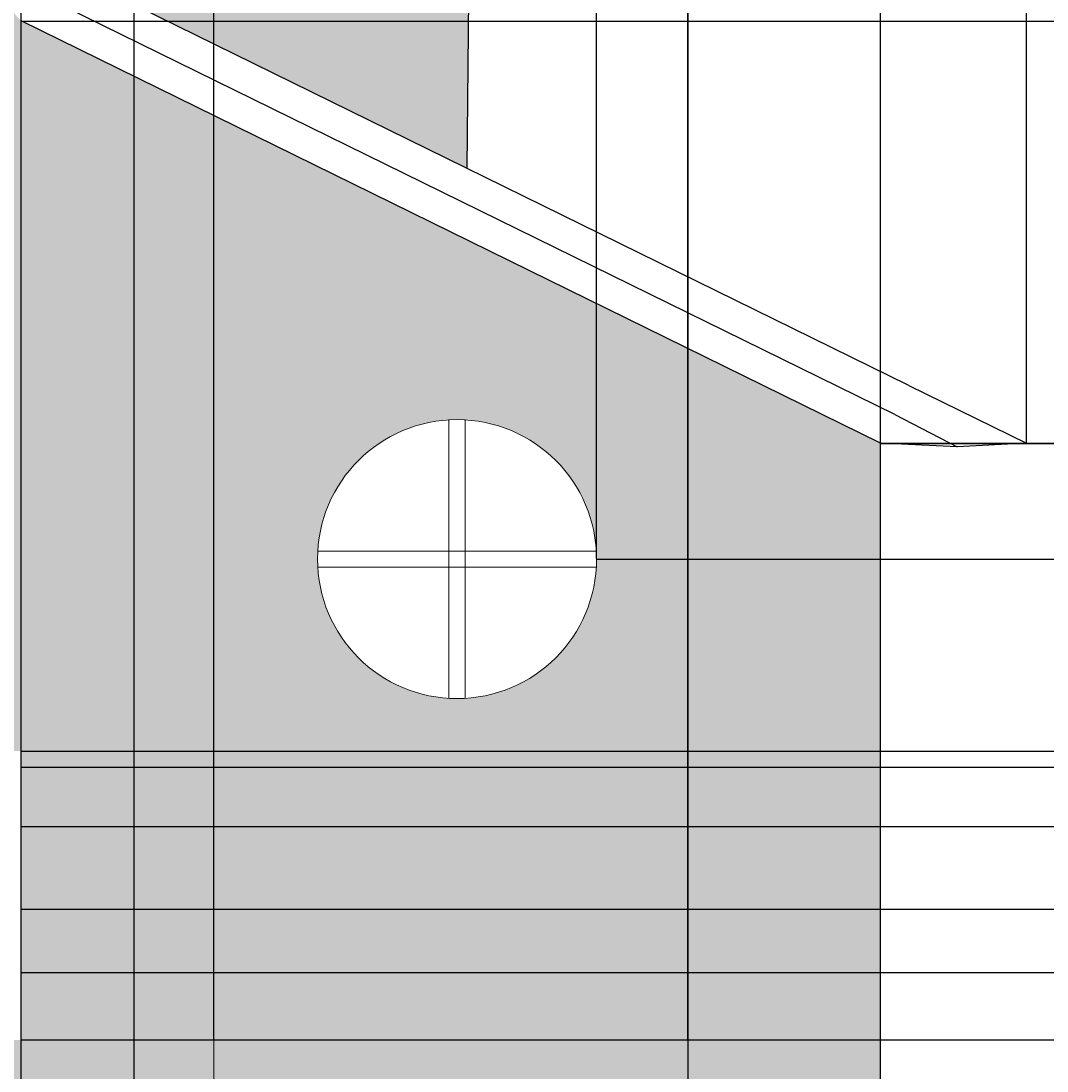
# Model space of a CAD drawing. Units: inches. Extents: x 36 to 594, y 79 to 831.
# Tile 27 of 30: x 342 to 469, y 590 to 721. Entities that reach past the tile are written whole.
import ezdxf

# ---------------------------------------------------------------- set-up
doc = ezdxf.new("R2010")
doc.units = ezdxf.units.IN
doc.header["$MEASUREMENT"] = 0
for name, color, linetype, lineweight in [('A-ANNO-DIMS', 2, 'Continuous', 18), ('A-ELEV', 7, 'Continuous', 25), ('A-ELEV-PATT', 8, 'Continuous', 13), ('A-GLAZ', 4, 'Continuous', 18)]:
    doc.layers.add(name, color=color, linetype=linetype, lineweight=lineweight)
doc.styles.get("Standard").update_dxf_attribs({"font": 'arial.ttf'})
doc.dimstyles.get("Standard").update_dxf_attribs({"dimtxt": 0.8125, "dimasz": 0.18, "dimexe": 0.18, "dimexo": 0.0625, "dimgap": 0.09, "dimtad": 0, "dimtih": 1, "dimtoh": 1, "dimdec": 4, "dimzin": 0, "dimdsep": 46, "dimlunit": 4, "dimtxsty": 'Standard', "dimcen": 0.09, "dimadec": 0, "dimazin": 0, "dimtfac": 1, "dimtdec": 4, "dimtofl": 0, "dimtmove": 0, "dimatfit": 3, "dimfxl": 1, "dimtolj": 1, "dimtzin": 0, "dimarcsym": 0})

# ---------------------------------------------------------------- blocks, each defined once
blk = doc.blocks.new('WIN-ROUND')
for p, q in [((146.46, 653.76), (146.46, 671.07)), ((148.46, 653.76), (148.46, 671.07)), ((147.46, 654.76), (130.16, 654.76)), ((147.46, 654.76), (164.77, 654.76)), ((147.46, 652.76), (130.16, 652.76)), ((146.46, 653.76), (146.46, 636.46)), ((147.46, 652.76), (164.77, 652.76)), ((148.46, 653.76), (148.46, 636.46))]:
    blk.add_line(p, q)
blk.add_circle((147.46, 653.76), 17.3)
blk = doc.blocks.new('*D18')
at = {"layer": 'A-ANNO-DIMS', "color": 0, "lineweight": -2, "transparency": 16777216}
for p, q in [((398.09, 796.11), (398.09, 830.73)), ((398.27, 830.55), (409.9, 830.55)), ((424.32, 830.55), (412.68, 830.55)), ((424.5, 594.27), (424.5, 830.73))]:
    blk.add_line(p, q, dxfattribs=at)
at = {"layer": 'A-ANNO-DIMS', "color": 0, "transparency": 16777216}
for points in [[(398.27, 830.58), (398.27, 830.52), (398.09, 830.55)], [(424.32, 830.58), (424.32, 830.52), (424.5, 830.55)]]:
    blk.add_solid(points, dxfattribs=at)
at = {"layer": 'Defpoints', "color": 0, "transparency": 16777216}
for p in [(424.5, 830.55), (398.09, 796.05), (424.5, 594.21)]:
    blk.add_point(p, dxfattribs=at)
at = {"layer": 'A-ANNO-DIMS', "color": 0, "transparency": 16777216, "insert": (411.29, 830.55), "char_height": 0.812, "attachment_point": 5}
blk.add_mtext('\\A1;26.41', dxfattribs=at)
blk = doc.blocks.new('*D19')
at = {"layer": 'A-ANNO-DIMS', "color": 0, "lineweight": -2, "transparency": 16777216}
for p, q in [((424.5, 594.27), (424.5, 830.73)), ((424.68, 830.55), (444.03, 830.55)), ((466.33, 830.55), (446.98, 830.55)), ((466.51, 668.28), (466.51, 830.73))]:
    blk.add_line(p, q, dxfattribs=at)
at = {"layer": 'A-ANNO-DIMS', "color": 0, "transparency": 16777216}
for points in [[(424.68, 830.58), (424.68, 830.52), (424.5, 830.55)], [(466.33, 830.58), (466.33, 830.52), (466.51, 830.55)]]:
    blk.add_solid(points, dxfattribs=at)
at = {"layer": 'Defpoints', "color": 0, "transparency": 16777216}
for p in [(466.51, 830.55), (466.51, 668.22), (424.5, 594.21)]:
    blk.add_point(p, dxfattribs=at)
at = {"layer": 'A-ANNO-DIMS', "color": 0, "transparency": 16777216, "insert": (445.5, 830.55), "char_height": 0.812, "attachment_point": 5}
blk.add_mtext('\\A1;42.02', dxfattribs=at)
blk = doc.blocks.new('*D20')
at = {"layer": 'A-ANNO-DIMS', "color": 0, "lineweight": -2, "transparency": 16777216}
for p, q in [((365.73, 594.27), (365.73, 830.73)), ((365.91, 830.55), (393.65, 830.55)), ((424.32, 830.55), (396.57, 830.55)), ((424.5, 594.27), (424.5, 830.73))]:
    blk.add_line(p, q, dxfattribs=at)
at = {"layer": 'A-ANNO-DIMS', "color": 0, "transparency": 16777216}
for points in [[(365.91, 830.58), (365.91, 830.52), (365.73, 830.55)], [(424.32, 830.58), (424.32, 830.52), (424.5, 830.55)]]:
    blk.add_solid(points, dxfattribs=at)
at = {"layer": 'Defpoints', "color": 0, "transparency": 16777216}
for p in [(424.5, 830.55), (365.73, 594.21), (424.5, 594.21)]:
    blk.add_point(p, dxfattribs=at)
at = {"layer": 'A-ANNO-DIMS', "color": 0, "transparency": 16777216, "insert": (395.11, 830.55), "char_height": 0.812, "attachment_point": 5}
blk.add_mtext('\\A1;58.77', dxfattribs=at)
blk = doc.blocks.new('*D24')
at = {"layer": 'A-ANNO-DIMS', "color": 0, "lineweight": -2, "transparency": 16777216}
for p, q in [((448.39, 668.27), (448.39, 830.73)), ((448.57, 830.55), (455.71, 830.55)), ((466.33, 830.55), (459.19, 830.55)), ((466.51, 668.28), (466.51, 830.73))]:
    blk.add_line(p, q, dxfattribs=at)
at = {"layer": 'A-ANNO-DIMS', "color": 0, "transparency": 16777216}
for points in [[(448.57, 830.58), (448.57, 830.52), (448.39, 830.55)], [(466.33, 830.58), (466.33, 830.52), (466.51, 830.55)]]:
    blk.add_solid(points, dxfattribs=at)
at = {"layer": 'Defpoints', "color": 0, "transparency": 16777216}
for p in [(466.51, 830.55), (448.39, 668.21), (466.51, 668.22)]:
    blk.add_point(p, dxfattribs=at)
at = {"layer": 'A-ANNO-DIMS', "color": 0, "transparency": 16777216, "insert": (457.45, 830.55), "char_height": 0.812, "attachment_point": 5}
blk.add_mtext('\\A1;18.123', dxfattribs=at)
blk = doc.blocks.new('*D35')
at = {"layer": 'A-ANNO-DIMS', "color": 0, "lineweight": -2, "transparency": 16777216}
for p, q in [((424.56, 594.21), (592.85, 594.21)), ((592.67, 594.03), (592.67, 522.71)), ((592.67, 450.39), (592.67, 521.71)), ((448.45, 450.21), (592.85, 450.21))]:
    blk.add_line(p, q, dxfattribs=at)
at = {"layer": 'A-ANNO-DIMS', "color": 0, "transparency": 16777216}
for points in [[(592.64, 594.03), (592.7, 594.03), (592.67, 594.21)], [(592.64, 450.39), (592.7, 450.39), (592.67, 450.21)]]:
    blk.add_solid(points, dxfattribs=at)
at = {"layer": 'Defpoints', "color": 0, "transparency": 16777216}
for p in [(424.5, 594.21), (592.67, 594.21), (448.39, 450.21)]:
    blk.add_point(p, dxfattribs=at)
at = {"layer": 'A-ANNO-DIMS', "color": 0, "transparency": 16777216, "insert": (592.67, 522.21), "char_height": 0.812, "attachment_point": 5}
blk.add_mtext('\\A1;144', dxfattribs=at)
blk = doc.blocks.new('*D36')
at = {"layer": 'A-ANNO-DIMS', "color": 0, "lineweight": -2, "transparency": 16777216}
for p, q in [((448.452274, 668.212359), (592.848908, 668.212359)), ((592.668908, 668.032359), (592.668908, 631.708609)), ((592.668908, 594.392359), (592.668908, 630.716109)), ((424.55834, 594.212359), (592.848908, 594.212359))]:
    blk.add_line(p, q, dxfattribs=at)
at = {"layer": 'A-ANNO-DIMS', "color": 0, "transparency": 16777216}
for points in [[(592.638908, 668.032359), (592.698908, 668.032359), (592.668908, 668.212359)], [(592.638908, 594.392359), (592.698908, 594.392359), (592.668908, 594.212359)]]:
    blk.add_solid(points, dxfattribs=at)
at = {"layer": 'Defpoints', "color": 0, "transparency": 16777216}
for p in [(448.389774, 668.212359), (592.668908, 668.212359), (424.49584, 594.212359)]:
    blk.add_point(p, dxfattribs=at)
at = {"layer": 'A-ANNO-DIMS', "color": 0, "transparency": 16777216, "insert": (592.668908, 631.212359), "char_height": 0.8125, "attachment_point": 5}
blk.add_mtext('\\A1;74', dxfattribs=at)
blk = doc.blocks.new('*D37')
at = {"layer": 'A-ANNO-DIMS', "color": 0, "lineweight": -2, "transparency": 16777216}
for p, q in [((330.04, 735.34), (592.85, 735.34)), ((592.67, 735.16), (592.67, 702.28)), ((592.67, 668.39), (592.67, 701.27)), ((448.45, 668.21), (592.85, 668.21))]:
    blk.add_line(p, q, dxfattribs=at)
at = {"layer": 'A-ANNO-DIMS', "color": 0, "transparency": 16777216}
for points in [[(592.64, 735.16), (592.7, 735.16), (592.67, 735.34)], [(592.64, 668.39), (592.7, 668.39), (592.67, 668.21)]]:
    blk.add_solid(points, dxfattribs=at)
at = {"layer": 'Defpoints', "color": 0, "transparency": 16777216}
for p in [(329.98, 735.34), (592.67, 735.34), (448.39, 668.21)]:
    blk.add_point(p, dxfattribs=at)
at = {"layer": 'A-ANNO-DIMS', "color": 0, "transparency": 16777216, "insert": (592.67, 701.77), "char_height": 0.812, "attachment_point": 5}
blk.add_mtext('\\A1;67.12', dxfattribs=at)
blk = doc.blocks.new('*D39')
at = {"layer": 'A-ANNO-DIMS', "color": 0, "lineweight": -2, "transparency": 16777216}
for p, q in [((413.2, 653.92), (413.2, 830.73)), ((413.38, 830.55), (429.02, 830.55)), ((448.21, 830.55), (432.57, 830.55)), ((448.39, 668.27), (448.39, 830.73))]:
    blk.add_line(p, q, dxfattribs=at)
at = {"layer": 'A-ANNO-DIMS', "color": 0, "transparency": 16777216}
for points in [[(413.38, 830.58), (413.38, 830.52), (413.2, 830.55)], [(448.21, 830.58), (448.21, 830.52), (448.39, 830.55)]]:
    blk.add_solid(points, dxfattribs=at)
at = {"layer": 'Defpoints', "color": 0, "transparency": 16777216}
for p in [(448.39, 830.55), (448.39, 668.21), (413.2, 653.86)]:
    blk.add_point(p, dxfattribs=at)
at = {"layer": 'A-ANNO-DIMS', "color": 0, "transparency": 16777216, "insert": (430.8, 830.55), "char_height": 0.812, "attachment_point": 5}
blk.add_mtext('\\A1;35.186', dxfattribs=at)
blk = doc.blocks.new('*D40')
at = {"layer": 'A-ANNO-DIMS', "color": 0, "lineweight": -2, "transparency": 16777216}
for p, q in [((413.27, 653.86), (592.85, 653.86)), ((592.67, 653.68), (592.67, 624.54)), ((592.67, 594.39), (592.67, 623.53)), ((424.56, 594.21), (592.85, 594.21))]:
    blk.add_line(p, q, dxfattribs=at)
at = {"layer": 'A-ANNO-DIMS', "color": 0, "transparency": 16777216}
for points in [[(592.64, 653.68), (592.7, 653.68), (592.67, 653.86)], [(592.64, 594.39), (592.7, 594.39), (592.67, 594.21)]]:
    blk.add_solid(points, dxfattribs=at)
at = {"layer": 'Defpoints', "color": 0, "transparency": 16777216}
for p in [(413.2, 653.86), (592.67, 653.86), (424.5, 594.21)]:
    blk.add_point(p, dxfattribs=at)
at = {"layer": 'A-ANNO-DIMS', "color": 0, "transparency": 16777216, "insert": (592.67, 624.03), "char_height": 0.812, "attachment_point": 5}
blk.add_mtext('\\A1;59.64', dxfattribs=at)
blk = doc.blocks.new('*D41')
at = {"layer": 'A-ANNO-DIMS', "color": 0, "lineweight": -2, "transparency": 16777216}
for p, q in [((341.9, 720.59), (592.85, 720.59)), ((592.67, 720.41), (592.67, 694.91)), ((592.67, 668.39), (592.67, 693.9)), ((448.45, 668.21), (592.85, 668.21))]:
    blk.add_line(p, q, dxfattribs=at)
at = {"layer": 'A-ANNO-DIMS', "color": 0, "transparency": 16777216}
for points in [[(592.64, 720.41), (592.7, 720.41), (592.67, 720.59)], [(592.64, 668.39), (592.7, 668.39), (592.67, 668.21)]]:
    blk.add_solid(points, dxfattribs=at)
at = {"layer": 'Defpoints', "color": 0, "transparency": 16777216}
for p in [(341.84, 720.59), (592.67, 720.59), (448.39, 668.21)]:
    blk.add_point(p, dxfattribs=at)
at = {"layer": 'A-ANNO-DIMS', "color": 0, "transparency": 16777216, "insert": (592.67, 694.4), "char_height": 0.812, "attachment_point": 5}
blk.add_mtext('\\A1;52.38', dxfattribs=at)
blk = doc.blocks.new('*D59')
at = {"layer": 'A-ANNO-DIMS', "color": 0, "lineweight": -2, "transparency": 16777216}
for p, q in [((355.86, 355.15), (355.86, 830.73)), ((356.04, 830.55), (388.74, 830.55)), ((424.37, 830.55), (391.67, 830.55)), ((424.55, 355.15), (424.55, 830.73))]:
    blk.add_line(p, q, dxfattribs=at)
at = {"layer": 'A-ANNO-DIMS', "color": 0, "transparency": 16777216}
for points in [[(356.04, 830.58), (356.04, 830.52), (355.86, 830.55)], [(424.37, 830.58), (424.37, 830.52), (424.55, 830.55)]]:
    blk.add_solid(points, dxfattribs=at)
at = {"layer": 'Defpoints', "color": 0, "transparency": 16777216}
for p in [(424.55, 830.55), (355.86, 355.08), (424.55, 355.08)]:
    blk.add_point(p, dxfattribs=at)
at = {"layer": 'A-ANNO-DIMS', "color": 0, "transparency": 16777216, "insert": (390.2, 830.55), "char_height": 0.812, "attachment_point": 5}
blk.add_mtext('\\A1;68.69', dxfattribs=at)
blk = doc.blocks.new('*D95')
at = {"layer": 'A-ANNO-DIMS', "color": 0, "lineweight": -2, "transparency": 16777216}
for p, q in [((260.51, 524.67), (260.51, 830.73)), ((260.69, 830.55), (299.71, 830.55)), ((341.66, 830.55), (302.63, 830.55)), ((341.84, 524.67), (341.84, 830.73))]:
    blk.add_line(p, q, dxfattribs=at)
at = {"layer": 'A-ANNO-DIMS', "color": 0, "transparency": 16777216}
for points in [[(260.69, 830.58), (260.69, 830.52), (260.51, 830.55)], [(341.66, 830.58), (341.66, 830.52), (341.84, 830.55)]]:
    blk.add_solid(points, dxfattribs=at)
at = {"layer": 'Defpoints', "color": 0, "transparency": 16777216}
for p in [(341.84, 830.55), (260.51, 524.6), (341.84, 524.6)]:
    blk.add_point(p, dxfattribs=at)
at = {"layer": 'A-ANNO-DIMS', "color": 0, "transparency": 16777216, "insert": (301.17, 830.55), "char_height": 0.812, "attachment_point": 5}
blk.add_mtext('\\A1;81.33', dxfattribs=at)
blk = doc.blocks.new('*D107')
at = {"layer": 'A-ANNO-DIMS', "color": 0, "lineweight": -2, "transparency": 16777216}
for p, q in [((269.04, 404.34), (269.04, 830.73)), ((269.22, 830.55), (310.99, 830.55)), ((355.68, 830.55), (313.91, 830.55)), ((355.86, 404.34), (355.86, 830.73))]:
    blk.add_line(p, q, dxfattribs=at)
at = {"layer": 'A-ANNO-DIMS', "color": 0, "transparency": 16777216}
for points in [[(269.22, 830.58), (269.22, 830.52), (269.04, 830.55)], [(355.68, 830.58), (355.68, 830.52), (355.86, 830.55)]]:
    blk.add_solid(points, dxfattribs=at)
at = {"layer": 'Defpoints', "color": 0, "transparency": 16777216}
for p in [(355.86, 830.55), (269.04, 404.27), (355.86, 404.27)]:
    blk.add_point(p, dxfattribs=at)
at = {"layer": 'A-ANNO-DIMS', "color": 0, "transparency": 16777216, "insert": (312.45, 830.55), "char_height": 0.812, "attachment_point": 5}
blk.add_mtext('\\A1;86.82', dxfattribs=at)
blk = doc.blocks.new('*D117')
at = {"layer": 'A-ANNO-DIMS', "color": 0, "lineweight": -2, "transparency": 16777216}
for p, q in [((341.9, 602.57), (592.85, 602.57)), ((592.67, 602.39), (592.67, 598.89)), ((592.67, 594.39), (592.67, 597.88)), ((341.9, 594.21), (592.85, 594.21))]:
    blk.add_line(p, q, dxfattribs=at)
at = {"layer": 'A-ANNO-DIMS', "color": 0, "transparency": 16777216}
for points in [[(592.64, 602.39), (592.7, 602.39), (592.67, 602.57)], [(592.64, 594.39), (592.7, 594.39), (592.67, 594.21)]]:
    blk.add_solid(points, dxfattribs=at)
at = {"layer": 'Defpoints', "color": 0, "transparency": 16777216}
for p in [(341.84, 602.57), (592.67, 602.57), (341.84, 594.21)]:
    blk.add_point(p, dxfattribs=at)
at = {"layer": 'A-ANNO-DIMS', "color": 0, "transparency": 16777216, "insert": (592.67, 598.39), "char_height": 0.812, "attachment_point": 5}
blk.add_mtext('\\A1;8.354', dxfattribs=at)
blk = doc.blocks.new('*D118')
at = {"layer": 'A-ANNO-DIMS', "color": 0, "lineweight": -2, "transparency": 16777216}
for p, q in [((341.9, 610.44), (592.85, 610.44)), ((592.67, 610.26), (592.67, 607.01)), ((592.67, 602.75), (592.67, 606)), ((341.9, 602.57), (592.85, 602.57))]:
    blk.add_line(p, q, dxfattribs=at)
at = {"layer": 'A-ANNO-DIMS', "color": 0, "transparency": 16777216}
for points in [[(592.64, 610.26), (592.7, 610.26), (592.67, 610.44)], [(592.64, 602.75), (592.7, 602.75), (592.67, 602.57)]]:
    blk.add_solid(points, dxfattribs=at)
at = {"layer": 'Defpoints', "color": 0, "transparency": 16777216}
for p in [(341.84, 610.44), (592.67, 610.44), (341.84, 602.57)]:
    blk.add_point(p, dxfattribs=at)
at = {"layer": 'A-ANNO-DIMS', "color": 0, "transparency": 16777216, "insert": (592.67, 606.5), "char_height": 0.812, "attachment_point": 5}
blk.add_mtext('\\A1;7.874', dxfattribs=at)
blk = doc.blocks.new('*D119')
at = {"layer": 'A-ANNO-DIMS', "color": 0, "lineweight": -2, "transparency": 16777216}
for p, q in [((341.9, 620.69), (592.85, 620.69)), ((592.67, 620.51), (592.67, 616.07)), ((592.67, 610.62), (592.67, 615.06)), ((341.9, 610.44), (592.85, 610.44))]:
    blk.add_line(p, q, dxfattribs=at)
at = {"layer": 'A-ANNO-DIMS', "color": 0, "transparency": 16777216}
for points in [[(592.64, 620.51), (592.7, 620.51), (592.67, 620.69)], [(592.64, 610.62), (592.7, 610.62), (592.67, 610.44)]]:
    blk.add_solid(points, dxfattribs=at)
at = {"layer": 'Defpoints', "color": 0, "transparency": 16777216}
for p in [(341.84, 620.69), (592.67, 620.69), (341.84, 610.44)]:
    blk.add_point(p, dxfattribs=at)
at = {"layer": 'A-ANNO-DIMS', "color": 0, "transparency": 16777216, "insert": (592.67, 615.56), "char_height": 0.812, "attachment_point": 5}
blk.add_mtext('\\A1;10.246', dxfattribs=at)
blk = doc.blocks.new('*D120')
at = {"layer": 'A-ANNO-DIMS', "color": 0, "lineweight": -2, "transparency": 16777216}
for p, q in [((341.9, 628.04), (592.85, 628.04)), ((592.67, 627.86), (592.67, 624.87)), ((592.67, 620.87), (592.67, 623.86)), ((341.9, 620.69), (592.85, 620.69))]:
    blk.add_line(p, q, dxfattribs=at)
at = {"layer": 'A-ANNO-DIMS', "color": 0, "transparency": 16777216}
for points in [[(592.64, 627.86), (592.7, 627.86), (592.67, 628.04)], [(592.64, 620.87), (592.7, 620.87), (592.67, 620.69)]]:
    blk.add_solid(points, dxfattribs=at)
at = {"layer": 'Defpoints', "color": 0, "transparency": 16777216}
for p in [(341.84, 628.04), (592.67, 628.04), (341.84, 620.69)]:
    blk.add_point(p, dxfattribs=at)
at = {"layer": 'A-ANNO-DIMS', "color": 0, "transparency": 16777216, "insert": (592.67, 624.36), "char_height": 0.812, "attachment_point": 5}
blk.add_mtext('\\A1;7.353', dxfattribs=at)
blk = doc.blocks.new('*D121')
at = {"layer": 'A-ANNO-DIMS', "color": 0, "lineweight": -2, "transparency": 16777216}
for p, q in [((341.9, 630.04), (592.85, 630.04)), ((592.67, 629.86), (592.67, 629.54)), ((341.9, 628.04), (592.85, 628.04)), ((592.67, 628.22), (592.67, 628.54))]:
    blk.add_line(p, q, dxfattribs=at)
at = {"layer": 'A-ANNO-DIMS', "color": 0, "transparency": 16777216}
for points in [[(592.64, 629.86), (592.7, 629.86), (592.67, 630.04)], [(592.64, 628.22), (592.7, 628.22), (592.67, 628.04)]]:
    blk.add_solid(points, dxfattribs=at)
at = {"layer": 'Defpoints', "color": 0, "transparency": 16777216}
for p in [(341.84, 630.04), (592.67, 630.04), (341.84, 628.04)]:
    blk.add_point(p, dxfattribs=at)
at = {"layer": 'A-ANNO-DIMS', "color": 0, "transparency": 16777216, "insert": (592.67, 629.04), "char_height": 0.812, "attachment_point": 5}
blk.add_mtext('\\A1;2', dxfattribs=at)
blk = doc.blocks.new('*D129')
at = {"layer": 'A-ANNO-DIMS', "color": 0, "lineweight": -2, "transparency": 16777216}
for p, q in [((316.05, 630.1), (316.05, 830.73)), ((316.23, 830.55), (327.16, 830.55)), ((341.66, 830.55), (330.73, 830.55)), ((341.84, 630.1), (341.84, 830.73))]:
    blk.add_line(p, q, dxfattribs=at)
at = {"layer": 'A-ANNO-DIMS', "color": 0, "transparency": 16777216}
for points in [[(316.23, 830.58), (316.23, 830.52), (316.05, 830.55)], [(341.66, 830.58), (341.66, 830.52), (341.84, 830.55)]]:
    blk.add_solid(points, dxfattribs=at)
at = {"layer": 'Defpoints', "color": 0, "transparency": 16777216}
for p in [(341.84, 830.55), (316.05, 630.04), (341.84, 630.04)]:
    blk.add_point(p, dxfattribs=at)
at = {"layer": 'A-ANNO-DIMS', "color": 0, "transparency": 16777216, "insert": (328.94, 830.55), "char_height": 0.812, "attachment_point": 5}
blk.add_mtext('\\A1;25.785', dxfattribs=at)

msp = doc.modelspace()

# ---------------------------------------------------------------- hatches: boundary and pattern name
at = {"layer": 'A-ELEV-PATT'}
h = msp.add_hatch(color=256, dxfattribs=at)
h.dxf.hatch_style = 1
h.paths.add_polyline_path([(398.0873, 796.0465), (269.3592, 796.0465), (269.3592, 770.1455), (397.8159, 770.1455)])
h.paths.add_polyline_path([(397.7518, 764.0341), (269.3592, 764.0341), (269.3592, 630.0394), (341.8367, 630.0394), (341.8367, 720.595), (335.0881, 728.3699), (329.982, 735.3373), (345.3661, 727.7743), (397.1052, 702.3389)])
h.paths.add_polyline_path([(341.8367, 594.2124), (201.4189, 594.2124), (201.4189, 475.4136), (232.8216, 475.4136), (232.8216, 524.6037), (341.8367, 524.6037)])
h.paths.add_polyline_path([(177.525, 594.2124), (118.7598, 594.2124), (118.7598, 450.2124), (177.525, 450.2124)])
h.paths.add_polyline_path([(424.4958, 594.2124), (365.7306, 594.2124), (365.7306, 450.2124), (424.4958, 450.2124)])
h.paths.add_polyline_path([(241.3553, 404.2737), (355.8569, 404.2737), (355.8569, 355.0836), (424.5492, 355.0836), (424.5492, 425.7333), (118.7598, 426.2844), (118.7598, 355.0836), (241.3553, 355.0836)])
h.paths.add_polyline_path([(448.3898, 306.2124), (217.0273, 306.2124), (217.0273, 142.2124), (254.0293, 142.2124), (254.0293, 150.9347), (254.0293, 286.1802), (401.5491, 286.1802), (401.5491, 150.9347), (401.5491, 142.2124), (448.3898, 142.2124)])
h.paths.add_polyline_path([(448.3898, 142.2124), (401.5491, 142.2124), (217.0273, 142.2124), (217.0273, 114.2124), (448.3898, 114.2124)])
h.paths.add_polyline_path([(217.0273, 306.2124), (174.7353, 306.2124), (94.8658, 306.2124), (94.8658, 162.2124), (103.3368, 162.2124), (103.3368, 264.6224), (103.3368, 286.1802), (217.0273, 286.1802)])
h = msp.add_hatch(color=256, dxfattribs=at)
h.dxf.hatch_style = 1
h.paths.add_polyline_path([(448.3898, 668.2124), (341.8367, 720.595), (341.8367, 594.2124), (341.8367, 450.2124), (365.7306, 450.2124), (365.7306, 594.2124), (424.4958, 594.2124), (424.4958, 450.2124), (448.3898, 450.2124), (448.3898, 594.2124)])
h.paths.add_polyline_path([(378.5958, 653.8563, -1), (413.2033, 653.8563, -1)], flags=16)
h.paths.add_polyline_path([(394.8995, 653.8563), (394.8995, 654.8563), (395.8995, 654.8563), (396.8995, 654.8563), (396.8995, 653.8563), (396.8995, 652.8563), (395.8995, 652.8563), (394.8995, 652.8563)], flags=0)
h.paths.add_polyline_path([(201.4189, 708.8485), (201.4189, 720.595), (94.8658, 668.2124), (94.8658, 644.2124), (94.8658, 596.2124), (94.8658, 594.2124), (94.8658, 450.2124), (118.7598, 450.2124), (118.7598, 594.2124), (177.525, 594.2124), (177.525, 450.2124), (201.4189, 450.2124), (201.4189, 594.2124)])
h.paths.add_polyline_path([(130.1589, 653.7648, -1), (164.7665, 653.7648, -1)], flags=16)
h.paths.add_polyline_path([(148.4627, 652.7648), (147.4627, 652.7648), (146.4627, 652.7648), (146.4627, 653.7648), (146.4627, 654.7648), (147.4627, 654.7648), (148.4627, 654.7648), (148.4627, 653.7648)], flags=0)

# ---------------------------------------------------------------- linework, layer by layer
at = {"layer": 'A-ELEV'}
for p, q in [((398.0873, 796.0465), (397.1052, 702.3389)), ((451.9192, 675.3917), (345.3661, 727.7743)), ((450.1545, 671.802), (343.6014, 724.1846)), ((448.3898, 668.2124), (341.8367, 720.595)), ((451.9192, 675.3917), (466.5128, 668.2174)), ((450.1545, 671.802), (457.8892, 667.7744)), ((448.3898, 594.2124), (448.3898, 668.2124)), ((457.8892, 667.7744), (448.3898, 668.2124)), ((466.5128, 668.2174), (457.8892, 667.7744)), ((448.3898, 450.2124), (448.3898, 594.2124))]:
    msp.add_line(p, q, dxfattribs=at)
at = {"layer": 'A-GLAZ'}
for p, q in [((365.7306, 450.2124), (365.7306, 594.2124)), ((365.7306, 594.2124), (424.4958, 594.2124)), ((424.4958, 450.2124), (424.4958, 594.2124))]:
    msp.add_line(p, q, dxfattribs=at)

# ---------------------------------------------------------------- block references
msp.add_blockref('WIN-ROUND', (248.4368, 0.0915), dxfattribs=at)

# ---------------------------------------------------------------- dimensions: what is measured, and where the dimension line sits
at = {"layer": 'A-ANNO-DIMS'}
for base, p1, p2, override, picture, middle in [((341.8367, 830.5465), (260.5056, 524.6037), (341.8367, 524.6037), {"dimdec": 2, "dimlfac": 1, "dimrnd": 0, "dimzin": 0, "dimdsep": 46, "dimlunit": 2}, '*D95', (301.1711, 830.5465)), ((355.8569, 830.5465), (269.0393, 404.2737), (355.8569, 404.2737), {"dimdec": 2, "dimlfac": 1, "dimrnd": 0, "dimzin": 0, "dimdsep": 46, "dimlunit": 2}, '*D107', (312.4481, 830.5465)), ((341.8367, 830.5465), (316.0513, 630.0394), (341.8367, 630.0394), {"dimdec": 3, "dimlfac": 1, "dimrnd": 0, "dimzin": 0, "dimdsep": 46, "dimlunit": 2}, '*D129', (328.944, 830.5465)), ((424.5492, 830.5465), (355.8569, 355.0836), (424.5492, 355.0836), {"dimdec": 2, "dimlfac": 1, "dimrnd": 0, "dimzin": 0, "dimdsep": 46, "dimlunit": 2}, '*D59', (390.203, 830.5465)), ((424.4958, 830.5465), (365.7306, 594.2124), (424.4958, 594.2124), {"dimdec": 2, "dimlfac": 1, "dimrnd": 0, "dimzin": 0, "dimdsep": 46, "dimlunit": 2}, '*D20', (395.1132, 830.5465)), ((424.4958, 830.5465), (398.0873, 796.0465), (424.4958, 594.2124), {"dimdec": 2, "dimlfac": 1, "dimrnd": 0, "dimzin": 0, "dimdsep": 46, "dimlunit": 2}, '*D18', (411.2916, 830.5465)), ((448.38977, 830.54647), (413.2033, 653.85634), (448.38977, 668.21236), {"dimdec": 3, "dimlfac": 1, "dimrnd": 0, "dimzin": 0, "dimdsep": 46, "dimlunit": 2}, '*D39', (430.79654, 830.54647)), ((466.5128, 830.5465), (424.4958, 594.2124), (466.5128, 668.2174), {"dimdec": 2, "dimlfac": 1, "dimrnd": 0, "dimzin": 0, "dimdsep": 46, "dimlunit": 2}, '*D19', (445.5043, 830.5465)), ((466.5128, 830.5465), (448.3898, 668.2124), (466.5128, 668.2174), {"dimdec": 3, "dimlfac": 1, "dimrnd": 0, "dimzin": 0, "dimdsep": 46, "dimlunit": 2}, '*D24', (457.4513, 830.5465))]:
    dim = msp.add_linear_dim(base=base, p1=p1, p2=p2, dimstyle='Standard', override=override, dxfattribs=at)
    dim.commit()
    dim.dimension.update_dxf_attribs({"geometry": picture, "text_midpoint": middle})
for base, p1, p2, override, picture, middle in [((592.6689, 735.3373), (448.3898, 668.2124), (329.982, 735.3373), {"dimdec": 2, "dimlfac": 1, "dimrnd": 0, "dimzin": 0, "dimdsep": 46, "dimlunit": 2}, '*D37', (592.6689, 701.7748)), ((592.6689, 720.595), (448.3898, 668.2124), (341.8367, 720.595), {"dimdec": 2, "dimlfac": 1, "dimrnd": 0, "dimzin": 0, "dimdsep": 46, "dimlunit": 2}, '*D41', (592.6689, 694.4037)), ((592.6689, 668.2124), (424.4958, 594.2124), (448.3898, 668.2124), {"dimdec": 0, "dimlfac": 1, "dimrnd": 0, "dimzin": 0, "dimdsep": 46, "dimlunit": 2}, '*D36', (592.6689, 631.2124)), ((592.6689, 653.8563), (424.4958, 594.2124), (413.2033, 653.8563), {"dimdec": 2, "dimlfac": 1, "dimrnd": 0, "dimzin": 0, "dimdsep": 46, "dimlunit": 2}, '*D40', (592.6689, 624.0344)), ((592.6689, 630.0394), (341.8367, 628.0394), (341.8367, 630.0394), {"dimdec": 0, "dimlfac": 1, "dimrnd": 0, "dimzin": 0, "dimdsep": 46, "dimlunit": 2}, '*D121', (592.6689, 629.0394)), ((592.6689, 628.0394), (341.8367, 620.6866), (341.8367, 628.0394), {"dimdec": 3, "dimlfac": 1, "dimrnd": 0, "dimzin": 0, "dimdsep": 46, "dimlunit": 2}, '*D120', (592.6689, 624.363)), ((592.6689, 620.6866), (341.8367, 610.4402), (341.8367, 620.6866), {"dimdec": 3, "dimlfac": 1, "dimrnd": 0, "dimzin": 0, "dimdsep": 46, "dimlunit": 2}, '*D119', (592.6689, 615.5634)), ((592.66891, 610.44025), (341.83669, 602.56672), (341.83669, 610.44025), {"dimdec": 3, "dimlfac": 1, "dimrnd": 0, "dimzin": 0, "dimdsep": 46, "dimlunit": 2}, '*D118', (592.66891, 606.50348)), ((592.6689, 602.5667), (341.8367, 594.2124), (341.8367, 602.5667), {"dimdec": 3, "dimlfac": 1, "dimrnd": 0, "dimzin": 0, "dimdsep": 46, "dimlunit": 2}, '*D117', (592.6689, 598.3895)), ((592.6689, 594.2124), (448.3898, 450.2124), (424.4958, 594.2124), {"dimdec": 0, "dimlfac": 1, "dimrnd": 0, "dimzin": 0, "dimdsep": 46, "dimlunit": 2}, '*D35', (592.6689, 522.2124))]:
    dim = msp.add_linear_dim(base=base, p1=p1, p2=p2, angle=90, dimstyle='Standard', override=override, dxfattribs=at)
    dim.commit()
    dim.dimension.update_dxf_attribs({"geometry": picture, "text_midpoint": middle})

doc.saveas('drawing.dxf')
